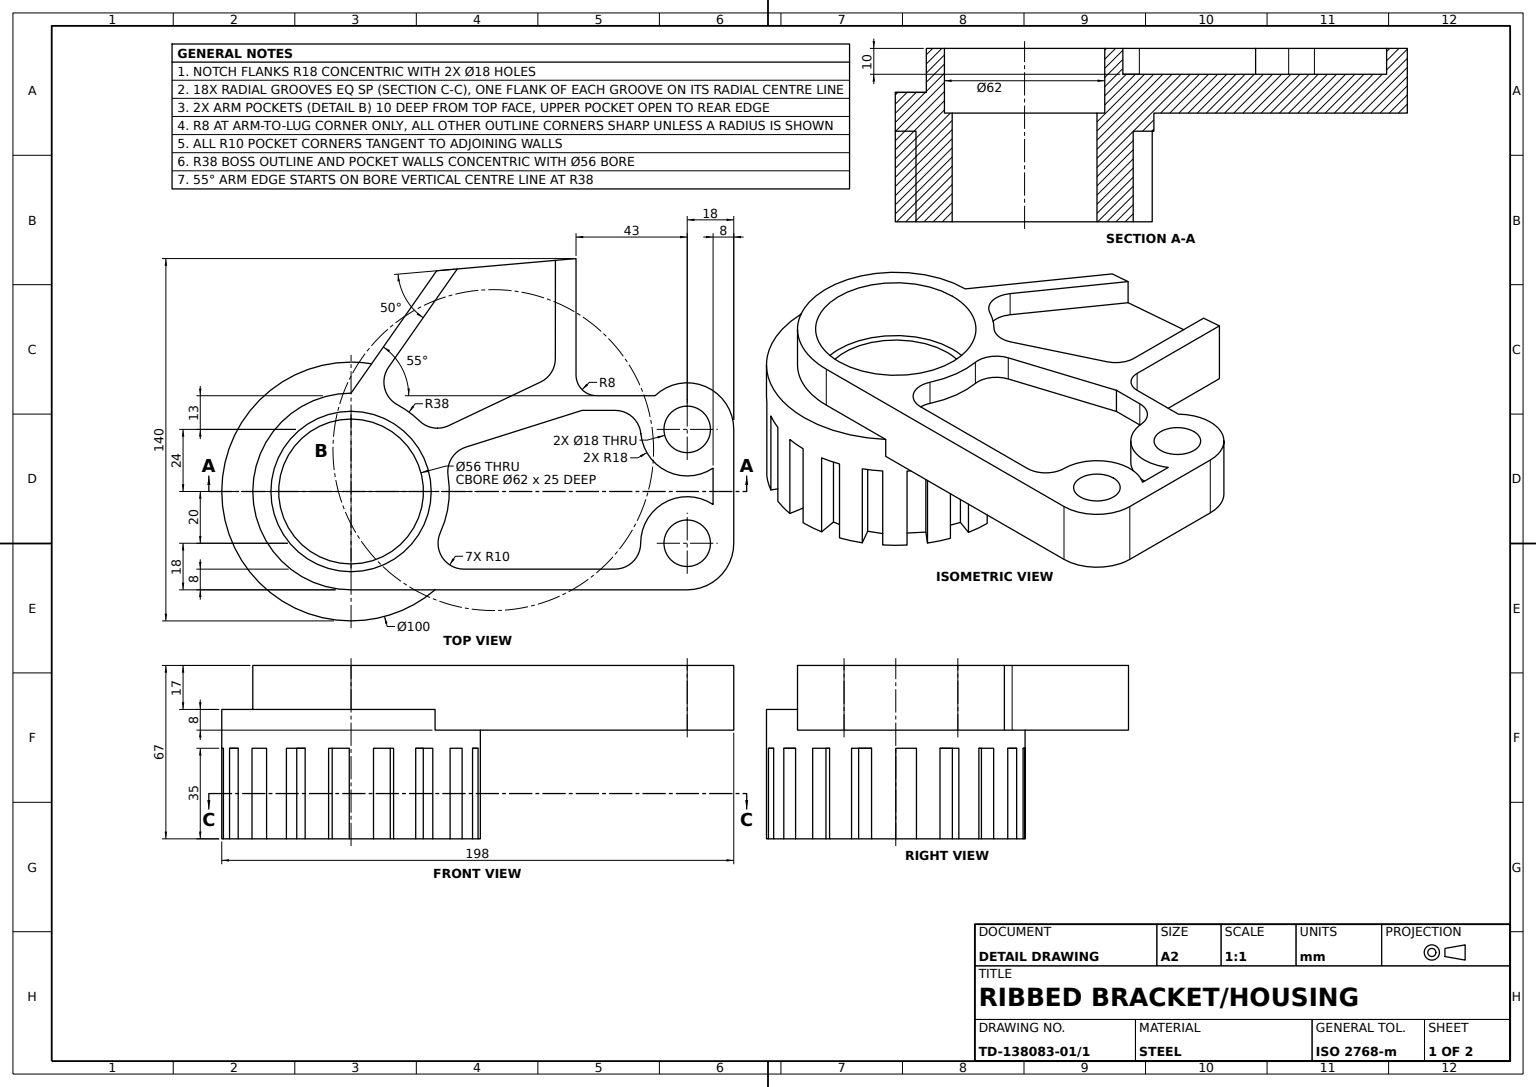
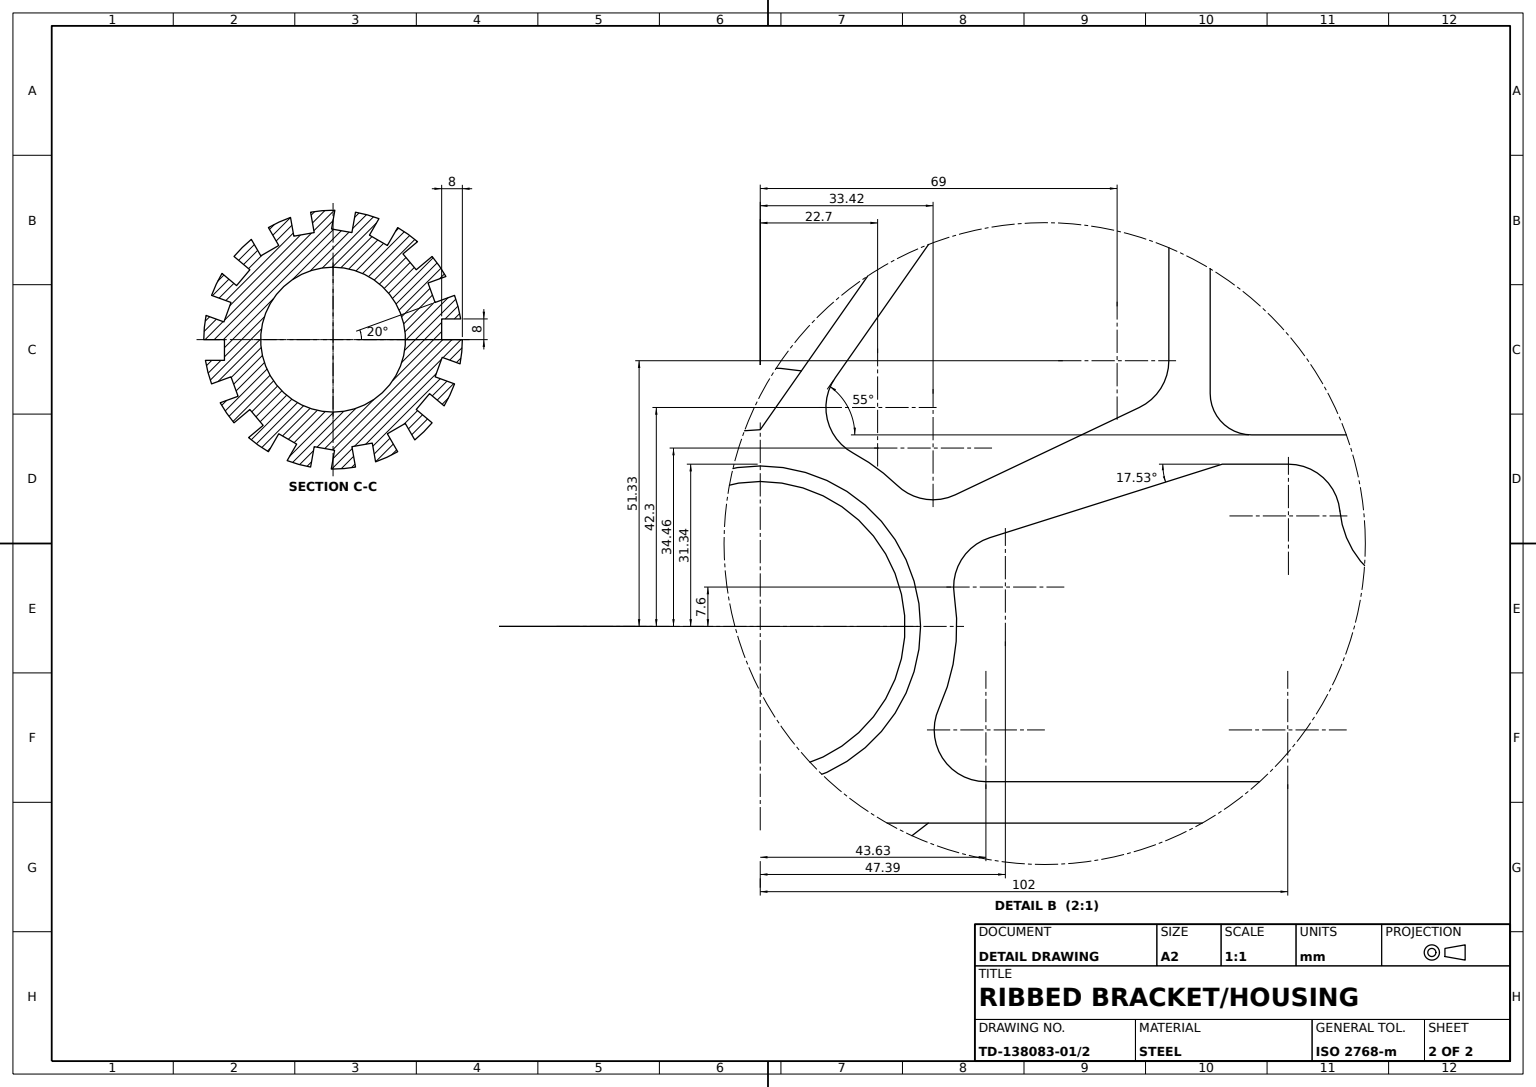
from build123d import *

# Parameters (mm, degrees)
HUB_PROFILE_SKETCH_R            = 50
HUB_CYLINDER_DEPTH              = 50
GROOVE_PROFILE_SKETCH_W         = 8
GROOVE_PROFILE_SKETCH_H         = 35
RADIAL_GROOVE_DEPTH             = 8
RADIAL_GROOVE_PATTERN_18X_COUNT = 18
BRACKET_ARM_DEPTH               = 17
BRACKET_ARM_DEPTH_BACK          = 8
BRACKET_ARM_SKETCH_R            = 9
ARM_START                       = -10
ARM_POCKETS_DEPTH               = 10
HUB_COUNTERBORE_SKETCH_R        = 31
HUB_COUNTERBORE_DEPTH           = 25
HUB_THROUGH_BORE_SKETCH_R       = 28
HUB_THROUGH_BORE_DEPTH          = 59
POCKET_FILLET_R10_A_R           = 10
POCKET_FILLET_R10_B_R           = 10
POCKET_FILLET_R10_C_R           = 10
POCKET_FILLET_R10_D_R           = 10
POCKET_FILLET_R10_E_R           = 10
POCKET_FILLET_R10_F_R           = 10
POCKET_FILLET_R10_G_R           = 10


with BuildPart() as part:
    # Hub Profile Sketch → Hub Cylinder (new body)
    with BuildSketch(Plane(origin=(0, 0, 0), x_dir=(1, 0, 0), z_dir=(0, 1, 0))):
        with Locations(Location((0, 0, 0), (0, 0, 270))):
            Circle(HUB_PROFILE_SKETCH_R)
    extrude(amount=HUB_CYLINDER_DEPTH)

    # Groove Profile Sketch → Radial Groove (cut)
    with BuildSketch(Plane(origin=(50, 0, 0), x_dir=(0, 0, -1), z_dir=(1, 0, 0))):
        with Locations((4, 17.5)):
            Rectangle(GROOVE_PROFILE_SKETCH_W, GROOVE_PROFILE_SKETCH_H)
    radial_groove = extrude(amount=-RADIAL_GROOVE_DEPTH, mode=Mode.SUBTRACT)

    # Radial Groove Pattern 18x: Radial Groove ×18 about axis
    radial_groove_pattern_18x_axis = Axis((0, 0, 0), (0, 1, 0))
    for i in range(1, RADIAL_GROOVE_PATTERN_18X_COUNT):
        add(radial_groove.rotate(radial_groove_pattern_18x_axis, i * 360 / RADIAL_GROOVE_PATTERN_18X_COUNT), mode=Mode.SUBTRACT)

    # Bracket Arm Sketch → Bracket Arm (add, two sides: drawn at the far end of the back side and taken through both)
    with BuildSketch(Plane(origin=(0, 50, 0), x_dir=(1, 0, 0), z_dir=(0, 1, 0)).offset(-BRACKET_ARM_DEPTH_BACK)):
        with BuildLine():
            Line((33.109444616, 85.285187333), (0, 38))
            ThreePointArc((0, 38), (-38, 0), (0, -38))
            Line((0, -38), (130, -38))
            ThreePointArc((130, -38), (142.727922061, -32.727922061), (148, -20))
            Line((148, -20), (148, 24))
            ThreePointArc((148, 24), (137.067595321, 40.554428301), (117.550100402, 37))
            Line((117.550100402, 37), (95, 37))
            ThreePointArc((95, 37), (89.343145751, 39.343145751), (87, 45))
            Line((87, 45), (87, 90))
            Line((87, 90), (33.109444616, 85.285187333))
        make_face()
        with Locations(Location((130, -20, 0), (0, 0, 270))):
            Circle(BRACKET_ARM_SKETCH_R, mode=Mode.SUBTRACT)
        with Locations(Location((130, 24, 0), (0, 0, 270))):
            Circle(BRACKET_ARM_SKETCH_R, mode=Mode.SUBTRACT)
    extrude(amount=BRACKET_ARM_DEPTH + BRACKET_ARM_DEPTH_BACK)

    # Arm Pocket Sketch → Arm Pockets (cut)
    with BuildSketch(Plane(origin=(0, 67, 0), x_dir=(1, 0, 0), z_dir=(0, 1, 0)).offset(ARM_START)):
        with BuildLine():
            ThreePointArc((38, 0), (34.134327941, -16.698732167), (23.323807579, -30))
            Line((23.323807579, -30), (65, -30))
            Line((65, -30), (115.033370453, -30))
            ThreePointArc((115.033370453, -30), (117.272077939, -7.272077939), (140, -5.033370453))
            Line((140, -5.033370453), (140, 2))
            Line((140, 2), (140, 9.033370453))
            ThreePointArc((140, 9.033370453), (118.390487135, 10.244302597), (113.565943578, 31.343145751))
            Line((113.565943578, 31.343145751), (89.343145751, 31.343145751))
            Line((89.343145751, 31.343145751), (35.229033551, 14.244830468))
            ThreePointArc((35.229033551, 14.244830468), (37.30082623, 7.255919138), (38, 0))
        make_face()
        with BuildLine():
            Line((79.030442415, 89.302754058), (41.079002201, 85.982433275))
            Line((41.079002201, 85.982433275), (7.022974779, 37.345385595))
            ThreePointArc((7.022974779, 37.345385595), (20.403319818, 32.057831187), (30.858927169, 22.17490956))
            Line((30.858927169, 22.17490956), (79, 45))
            Line((79, 45), (79.030442415, 89.302754058))
        make_face()
    extrude(amount=ARM_POCKETS_DEPTH, mode=Mode.SUBTRACT)

    # Hub Counterbore Sketch → Hub Counterbore (cut)
    with BuildSketch(Plane(origin=(0, 67, 0), x_dir=(1, 0, 0), z_dir=(0, 1, 0))):
        with Locations(Location((0, 0, 0), (0, 0, 270))):
            Circle(HUB_COUNTERBORE_SKETCH_R)
    extrude(amount=-HUB_COUNTERBORE_DEPTH, mode=Mode.SUBTRACT)

    # Hub Through Bore Sketch → Hub Through Bore (cut)
    with BuildSketch(Plane(origin=(0, 42, 0), x_dir=(1, 0, 0), z_dir=(0, 1, 0))):
        with Locations(Location((0, 0, 0), (0, 0, 270))):
            Circle(HUB_THROUGH_BORE_SKETCH_R)
    extrude(amount=-HUB_THROUGH_BORE_DEPTH, mode=Mode.SUBTRACT)

    # Pocket Fillet R10 A
    pocket_fillet_r10_a_edges = [part.edges().sort_by_distance(p)[0] for p in [
        (23.323807579, 62, 30),
    ]]
    fillet(pocket_fillet_r10_a_edges, radius=POCKET_FILLET_R10_A_R)

    # Pocket Fillet R10 B
    pocket_fillet_r10_b_edges = [part.edges().sort_by_distance(p)[0] for p in [
        (115.033370453, 62, 30),
    ]]
    fillet(pocket_fillet_r10_b_edges, radius=POCKET_FILLET_R10_B_R)

    # Pocket Fillet R10 C
    pocket_fillet_r10_c_edges = [part.edges().sort_by_distance(p)[0] for p in [
        (113.565943578, 62, -31.343145751),
    ]]
    fillet(pocket_fillet_r10_c_edges, radius=POCKET_FILLET_R10_C_R)

    # Pocket Fillet R10 D
    pocket_fillet_r10_d_edges = [part.edges().sort_by_distance(p)[0] for p in [
        (35.229033551, 62, -14.244830468),
    ]]
    fillet(pocket_fillet_r10_d_edges, radius=POCKET_FILLET_R10_D_R)

    # Pocket Fillet R10 E
    pocket_fillet_r10_e_edges = [part.edges().sort_by_distance(p)[0] for p in [
        (30.858927169, 62, -22.17490956),
    ]]
    fillet(pocket_fillet_r10_e_edges, radius=POCKET_FILLET_R10_E_R)

    # Pocket Fillet R10 F
    pocket_fillet_r10_f_edges = [part.edges().sort_by_distance(p)[0] for p in [
        (79, 62, -45),
    ]]
    fillet(pocket_fillet_r10_f_edges, radius=POCKET_FILLET_R10_F_R)

    # Pocket Fillet R10 G
    pocket_fillet_r10_g_edges = [part.edges().sort_by_distance(p)[0] for p in [
        (7.022974779, 62, -37.345385595),
    ]]
    fillet(pocket_fillet_r10_g_edges, radius=POCKET_FILLET_R10_G_R)


solid = part.part
